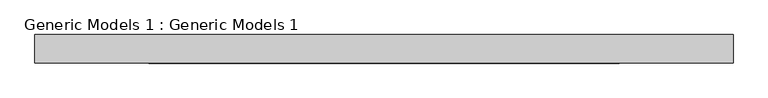
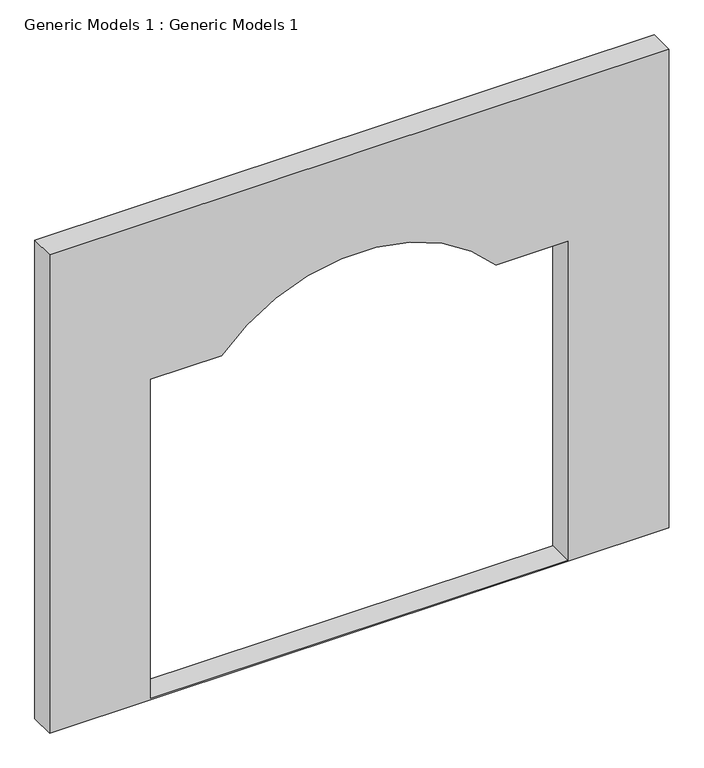
"""IFC4 building model written with IfcOpenShell, lengths in millimetres: proxy geometry, Generic Models 1 : Generic Models 1."""

from ifc_helpers import new_model, si_unit, point, frame, frame_2d, origin, place, context, project, spatial, polyline, circle_curve, trimmed, segment, composite_curve, outline, extrude, source, transform, mapped, element, save


def generic_models_1_generic_models_1_99b3fc70(model_context):
    return source(origin(), model_context, "Body", "SweptSolid", [
        extrude(outline(polyline([(3352.8, -7911.9236584), (3352.8, -11645.7236584), (304.8, -11645.7236584), (304.8, -7911.9236584), (3352.8, -7911.9236584)]), holes=[composite_curve([segment(polyline([(2343.9330823, -11036.1236584), (2343.9330823, -10604.3236584)]), True, "CONTINUOUS"), segment(trimmed(circle_curve(frame_2d((1611.4465902, -9778.8236584)), 1103.6243524), [point((2343.9330823, -10604.3236584))], [point((2343.9330823, -8953.3236584))], True, "CARTESIAN"), True, "CONTINUOUS"), segment(polyline([(2343.9330823, -8953.3236584), (2343.9330823, -8521.5236584), (312.5949901, -8521.5236584), (312.5949901, -11036.1236584), (2343.9330823, -11036.1236584)]), True, "CONTINUOUS")], self_intersect=False)]), frame((0.0, -13640.202305, 0.0), z_axis=(0.0, 1.0, 0.0), x_axis=(0.0, 0.0, 1.0)), (0.0, 0.0, 1.0), 152.4),
    ])


if __name__ == "__main__":
    model = new_model("IFC4")
    model_context = context("Model", 3, world=origin())
    ifc_project = project(units=[si_unit("LENGTHUNIT", "METRE", prefix="MILLI")], contexts=[model_context])
    site = spatial("IfcSite", under=ifc_project)
    building = spatial("IfcBuilding", under=site)
    placement = place(None, origin())
    generic_models_1_generic_models_1_shape = generic_models_1_generic_models_1_99b3fc70(model_context)
    element("IfcBuildingElementProxy", 1, Name="Generic Models 1 : Generic Models 1", ObjectType="Generic Models 1 : Generic Models 1", at=placement, inside=building, context=model_context, shape_type="MappedRepresentation", body=[
        mapped(generic_models_1_generic_models_1_shape, transform((0.0, 0.0, 0.0), x_axis=(1.0, 0.0, 0.0), y_axis=(0.0, 1.0, 0.0), z_axis=(0.0, 0.0, 1.0))),
    ])
    save(model, "model.ifc")

# Revit data of these elements
# Element 1 (IfcBuildingElementProxy, "Generic Models 1 : Generic Models 1")
#   Materials on its faces: "ACCENT BEIGE COLOUR"
# Materials
#   "ACCENT BEIGE COLOUR": class "Generic", colour RGB 120 120 120, transparency 0, Cost = 0
